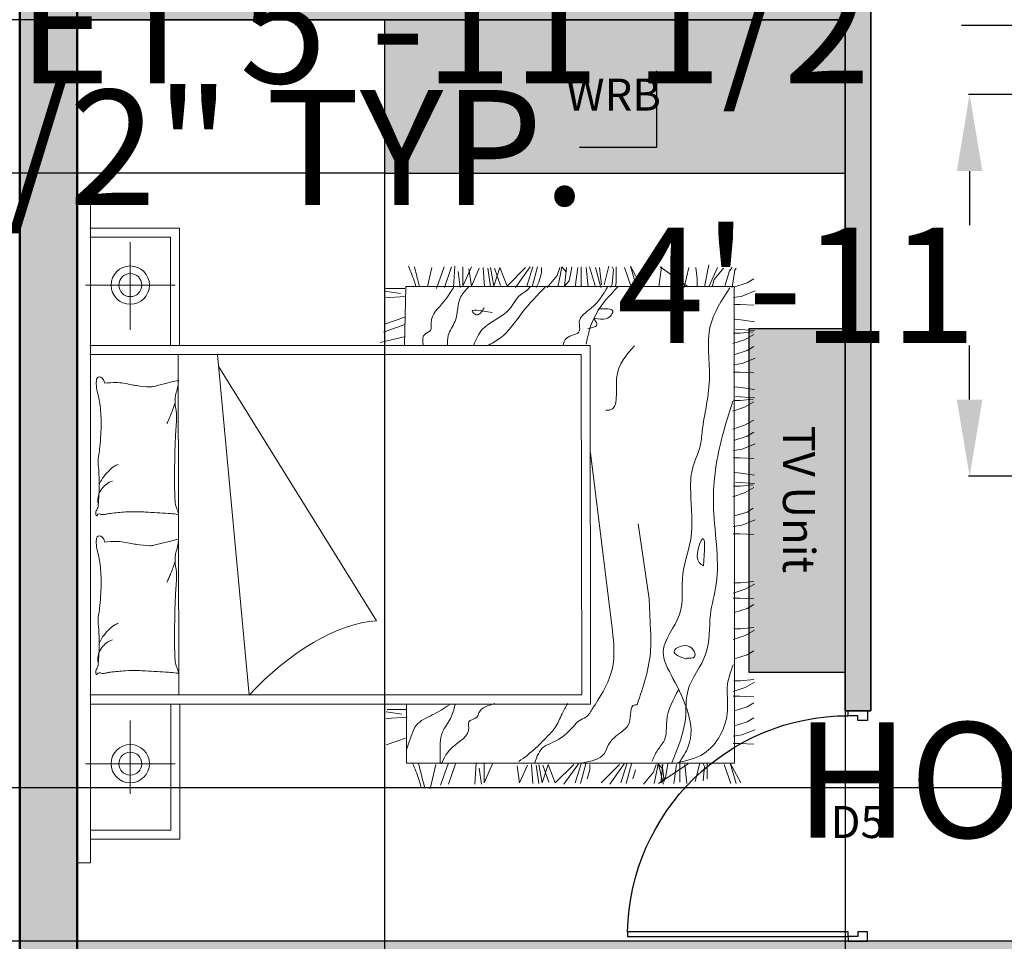
# Model space of a CAD drawing. Units: inches. Extents: x 2796 to 3603, y 978 to 1787.
# Tile 8 of 15: x 3070 to 3224, y 1312 to 1456. Entities that reach past the tile are written whole.
import ezdxf

# ---------------------------------------------------------------- set-up
doc = ezdxf.new("R2010")
doc.units = ezdxf.units.IN
for name, color, linetype, lineweight in [('A-ANNO-DIMS', 7, 'Continuous', 18), ('A-ANNO-TEXT', 7, 'Continuous', 18), ('A-DOOR', 6, 'Continuous', 25), ('A-FLOR-CASE', 2, 'Continuous', 25), ('A-FLOR-CASE-PATT', 2, 'Continuous', 13), ('A-WALL-EXTR-PATT', 1, 'Continuous', 13), ('A-WALL-INTR-PATT', 5, 'Continuous', 13), ('Furniture', 2, 'Continuous', 18), ('Inner Wall', 5, 'Continuous', 35), ('Outer Wall', 1, 'Continuous', 50)]:
    doc.layers.add(name, color=color, linetype=linetype, lineweight=lineweight)
doc.styles.get("Standard").update_dxf_attribs({"font": 'arial.ttf'})
doc.dimstyles.get("Standard").update_dxf_attribs({"dimtxt": 18, "dimasz": 12, "dimexe": 0.18, "dimexo": 0.0625, "dimgap": 0.09, "dimtad": 0, "dimtih": 1, "dimtoh": 1, "dimdec": 0, "dimzin": 0, "dimdsep": 46, "dimlunit": 3, "dimtxsty": 'Standard', "dimcen": 0.09, "dimadec": 0, "dimazin": 0, "dimtfac": 1, "dimtdec": 0, "dimtofl": 0, "dimtmove": 0, "dimatfit": 3, "dimfxl": 1, "dimtolj": 1, "dimtzin": 0, "dimarcsym": 0})

# ---------------------------------------------------------------- blocks, each defined once
blk = doc.blocks.new('A$C2B723114')
for p, q in [((0, 2.9047), (2.8274, 2.9047)), ((0, 2.8487), (0, 2.9047)), ((0.4243, 2.8697), (0.4243, 2.4855)), ((2.4742, 2.8697), (2.4742, 2.4855)), ((2.8274, 2.9047), (2.8274, 2.8487)), ((2.8274, 2.8487), (0, 2.8487)), ((0.1012, 2.4649), (0.1012, 2.849)), ((0.1396, 2.5033), (0.1396, 2.849)), ((0.6794, 0.7051), (0.6794, 2.8509)), ((0.7187, 0.7435), (0.7187, 2.8509)), ((2.1776, 2.8509), (2.1776, 0.7454)), ((2.216, 2.8509), (2.216, 0.707)), ((2.6798, 2.5052), (2.6798, 2.8509)), ((2.7182, 2.4668), (2.7182, 2.8509)), ((0.6087, 2.6776), (0.295, 2.6776)), ((2.6586, 2.6776), (2.2821, 2.6776)), ((1.3789, 2.4999), (1.3598, 2.5761)), ((2.0593, 2.4999), (2.0402, 2.5761)), ((0.6766, 2.5033), (0.1396, 2.5033)), ((1.3858, 2.4723), (1.3789, 2.4999)), ((2.0662, 2.4723), (2.0593, 2.4999)), ((2.2188, 2.5052), (2.6798, 2.5052)), ((0.6794, 2.4649), (0.1012, 2.4649)), ((0.7191, 2.47), (2.1778, 2.4719)), ((2.2188, 2.4668), (2.7182, 2.4668)), ((2.1771, 2.3036), (0.718, 2.1685)), ((1.0365, 1.6233), (2.1246, 2.2989)), ((2.2287, 1.6076), (2.2523, 1.5035)), ((0.5047, 1.5819), (0.5353, 1.4945)), ((0.6174, 1.5819), (0.6232, 1.4916)), ((0.6467, 1.5819), (0.6369, 1.5137)), ((0.6571, 1.4945), (0.6571, 1.5765)), ((2.2726, 1.593), (2.3061, 1.5007)), ((2.3067, 1.5881), (2.3373, 1.5007)), ((2.4194, 1.5881), (2.4251, 1.4979)), ((2.4487, 1.5881), (2.4389, 1.5199)), ((2.4591, 1.5007), (2.4591, 1.5828)), ((0.4269, 0.0884), (0.4269, 1.4945)), ((0.4269, 1.4945), (0.6794, 1.4945)), ((2.4685, 1.4964), (2.216, 1.5022)), ((2.4685, 1.4964), (2.4685, 0.0903)), ((0.3172, 1.3923), (0.4213, 1.3687)), ((2.4685, 1.4044), (2.5491, 1.3861)), ((2.4596, 1.3659), (2.552, 1.3324)), ((0.3318, 1.3485), (0.4241, 1.3149)), ((0.3367, 1.3143), (0.4241, 1.2838)), ((2.4645, 1.3318), (2.552, 1.3012)), ((2.4645, 1.2928), (2.5548, 1.2871)), ((2.4645, 1.2635), (2.5328, 1.2733)), ((2.4699, 1.2531), (2.552, 1.2163)), ((2.552, 1.2531), (2.4699, 1.2531)), ((2.5435, 1.2276), (2.4699, 1.2163)), ((0.3367, 1.2016), (0.427, 1.1959)), ((0.3367, 1.1724), (0.405, 1.1821)), ((2.4699, 1.2163), (2.5463, 1.1823)), ((0.4241, 1.162), (0.3421, 1.162)), ((0.3421, 1.162), (0.4241, 1.1252)), ((2.5491, 1.1654), (2.467, 1.1597)), ((2.5463, 1.1455), (2.467, 1.1342)), ((2.5491, 1.1342), (2.4699, 1.1201)), ((2.4699, 1.1201), (2.5491, 1.0946)), ((2.5463, 1.1172), (2.4727, 1.0918)), ((2.5491, 1.0946), (2.4699, 1.0635)), ((2.4699, 1.0635), (2.5491, 0.9842)), ((0.4157, 1.0206), (0.3421, 1.0093)), ((2.4642, 1.0267), (2.552, 0.9644)), ((0.3421, 1.0093), (0.4185, 0.9754)), ((2.4699, 0.9785), (2.552, 0.9531)), ((0.4213, 0.9584), (0.3392, 0.9527)), ((0.4185, 0.9386), (0.3392, 0.9272)), ((2.4642, 0.9389), (2.4869, 0.9276)), ((2.467, 0.9559), (2.552, 0.9333)), ((0.4213, 0.9272), (0.3421, 0.9131)), ((0.3421, 0.9131), (0.4213, 0.8876)), ((0.4213, 0.8876), (0.3421, 0.8565)), ((0.4185, 0.9103), (0.3449, 0.8848)), ((2.4642, 0.8908), (2.5152, 0.8483)), ((2.4869, 0.9276), (2.5265, 0.9163)), ((2.5265, 0.9163), (2.5491, 0.9163)), ((0.3421, 0.8565), (0.4213, 0.7772)), ((2.467, 0.8455), (2.5208, 0.8342)), ((2.5152, 0.8483), (2.5491, 0.837)), ((0.3364, 0.8197), (0.4241, 0.7574)), ((2.4699, 0.8172), (2.4925, 0.7974)), ((2.5491, 0.8087), (2.4699, 0.8172)), ((2.5208, 0.8342), (2.552, 0.8285)), ((2.552, 0.8285), (2.5293, 0.8087)), ((0.3421, 0.7716), (0.4241, 0.7461)), ((2.5491, 0.7606), (2.467, 0.7719)), ((2.4925, 0.7974), (2.535, 0.7889)), ((2.535, 0.7889), (2.552, 0.7861)), ((0.3392, 0.7489), (0.4241, 0.7263)), ((0.359, 0.7206), (0.3987, 0.7093)), ((2.1776, 0.7454), (0.7187, 0.7435)), ((2.4727, 0.7464), (2.467, 0.7408)), ((2.467, 0.7153), (2.5491, 0.7238)), ((2.552, 0.7464), (2.4727, 0.7464)), ((0.3987, 0.7093), (0.4213, 0.7093)), ((2.216, 0.707), (0.6794, 0.7051)), ((0.9938, 0.6115), (1.7555, 0.7064)), ((2.5491, 0.6842), (2.4642, 0.6615)), ((2.552, 0.7096), (2.467, 0.6842)), ((0.3421, 0.6601), (0.4213, 0.5808)), ((2.5491, 0.6672), (2.4755, 0.6587)), ((2.4755, 0.6474), (2.5548, 0.6276)), ((0.3364, 0.6233), (0.4241, 0.561)), ((2.4642, 0.6191), (2.4784, 0.6134)), ((2.467, 0.5993), (2.4869, 0.5964)), ((2.4784, 0.6134), (2.5406, 0.6077)), ((2.4869, 0.5964), (2.552, 0.5964)), ((2.5406, 0.6077), (2.552, 0.6134)), ((0.3392, 0.5525), (0.4241, 0.5299)), ((0.3421, 0.5752), (0.4241, 0.5497)), ((2.467, 0.5313), (2.5491, 0.5596)), ((0.359, 0.5242), (0.3987, 0.5129)), ((2.467, 0.5087), (2.5548, 0.5342)), ((2.5548, 0.5342), (2.4699, 0.4889)), ((0.3364, 0.4785), (0.3874, 0.436)), ((1.4523, 0.5021), (1.1305, 0.4537)), ((0.3392, 0.4332), (0.393, 0.4219)), ((0.3874, 0.436), (0.4213, 0.4247)), ((1.1305, 0.4537), (0.9938, 0.448)), ((0.4213, 0.415), (0.3364, 0.3923)), ((0.4241, 0.2868), (0.3392, 0.415)), ((0.3421, 0.4049), (0.3647, 0.3851)), ((0.4213, 0.3964), (0.3421, 0.4049)), ((0.4213, 0.398), (0.3477, 0.3895)), ((0.3647, 0.3851), (0.4072, 0.3766)), ((0.393, 0.4219), (0.4241, 0.4162)), ((0.4241, 0.4162), (0.4015, 0.3964)), ((2.467, 0.4133), (2.552, 0.4019)), ((2.467, 0.2879), (2.552, 0.4076)), ((0.4213, 0.3377), (0.3392, 0.3491)), ((0.4072, 0.3766), (0.4241, 0.3738)), ((0.3392, 0.2925), (0.4213, 0.3009)), ((0.4241, 0.3236), (0.3449, 0.3236)), ((2.4642, 0.3049), (2.5491, 0.2851)), ((2.467, 0.319), (2.5548, 0.3134)), ((0.3477, 0.2571), (0.427, 0.2373)), ((2.501, 0.2491), (2.5491, 0.2547)), ((0.3506, 0.2231), (0.4128, 0.2175)), ((0.4128, 0.2175), (0.4241, 0.2231)), ((2.467, 0.2179), (2.5605, 0.1981)), ((2.4699, 0.2491), (2.501, 0.2491)), ((0.359, 0.2061), (0.4241, 0.2061)), ((2.467, 0.1981), (2.5491, 0.1613)), ((2.467, 0.184), (2.4982, 0.1755)), ((2.4982, 0.1755), (2.5463, 0.1359)), ((0.3392, 0.1042), (0.4213, 0.1325)), ((2.4699, 0.1302), (2.535, 0.1104)), ((0.3392, 0.0815), (0.427, 0.107)), ((0.427, 0.107), (0.3421, 0.0617)), ((2.4685, 0.0903), (0.4269, 0.0884)), ((0.5106, 0.094), (0.5106, 0.0657)), ((0.5417, 0.094), (0.5474, 0.0572)), ((0.587, 0.0884), (0.604, 0.0346)), ((0.6512, 0.0884), (0.6682, 0.0346)), ((0.713, 0.094), (0.713, 0.0657)), ((0.7334, 0.0943), (0.7503, 0.0434)), ((0.7786, 0.0915), (0.7786, 0.0632)), ((0.8739, 0.0884), (0.8908, 0.0346)), ((0.956, 0.0943), (0.973, 0.0434)), ((1.0013, 0.0915), (1.0013, 0.0632)), ((1.072, 0.0884), (1.089, 0.0346)), ((1.1338, 0.094), (1.1338, 0.0657)), ((1.1542, 0.0943), (1.1712, 0.0434)), ((1.1995, 0.0915), (1.1995, 0.0632)), ((1.4088, 0.094), (1.4088, 0.0657)), ((1.44, 0.094), (1.4456, 0.0572)), ((1.4853, 0.0884), (1.5023, 0.0346)), ((1.5674, 0.0962), (1.5844, 0.0453)), ((1.6127, 0.0934), (1.6127, 0.0651)), ((1.6297, 0.0849), (1.624, 0.0028)), ((1.6721, 0.0877), (1.6693, 0.0623)), ((1.7344, 0.0934), (1.7344, 0.0651)), ((1.7655, 0.0934), (1.7712, 0.0566)), ((1.8108, 0.0877), (1.8278, 0.034)), ((1.8568, 0.0962), (1.8738, 0.0453)), ((1.9342, 0.0962), (1.9512, 0.0453)), ((1.9795, 0.0934), (1.9795, 0.0651)), ((1.9965, 0.0849), (1.9908, 0.0028)), ((2.039, 0.0877), (2.0361, 0.0623)), ((2.1012, 0.0934), (2.1012, 0.0651)), ((2.1324, 0.0934), (2.138, 0.0566)), ((2.1777, 0.0877), (2.1946, 0.034)), ((2.2236, 0.0962), (2.2406, 0.0453)), ((2.2689, 0.0934), (2.2689, 0.0651)), ((2.2859, 0.0849), (2.2802, 0.0028)), ((2.3284, 0.0877), (2.3255, 0.0623)), ((2.3906, 0.0934), (2.3906, 0.0651)), ((2.4218, 0.0934), (2.4274, 0.0566)), ((2.4642, 0.0991), (2.5378, 0.0877)), ((2.467, 0.0877), (2.484, 0.034)), ((2.535, 0.1104), (2.5491, 0.0991)), ((2.5378, 0.0877), (2.5463, 0.0821)), ((0.5106, 0.0657), (0.5077, 0.0063)), ((0.5474, 0.0572), (0.57, 0.0006)), ((0.713, 0.0657), (0.7101, 0.0063)), ((0.7503, 0.0434), (0.773, 0.0037)), ((0.7786, 0.0632), (0.7843, 0.0066)), ((0.973, 0.0434), (0.9957, 0.0037)), ((1.0013, 0.0632), (1.007, 0.0066)), ((1.1338, 0.0657), (1.131, 0.0063)), ((1.1712, 0.0434), (1.1939, 0.0037)), ((1.1995, 0.0632), (1.2052, 0.0066)), ((1.4088, 0.0657), (1.406, 0.0063)), ((1.4456, 0.0572), (1.4683, 0.0006)), ((1.5844, 0.0453), (1.607, 0.0057)), ((1.6127, 0.0651), (1.6184, 0.0085)), ((1.6693, 0.0623), (1.6608, 0.0028)), ((1.7344, 0.0651), (1.7316, 0.0057)), ((1.7712, 0.0566), (1.7938, 0)), ((1.8738, 0.0453), (1.8964, 0.0057)), ((1.9512, 0.0453), (1.9739, 0.0057)), ((1.9795, 0.0651), (1.9852, 0.0085)), ((2.0361, 0.0623), (2.0276, 0.0028)), ((2.1012, 0.0651), (2.0984, 0.0057)), ((2.138, 0.0566), (2.1607, 0)), ((2.2406, 0.0453), (2.2632, 0.0057)), ((2.2689, 0.0651), (2.2746, 0.0085)), ((2.3255, 0.0623), (2.317, 0.0028)), ((2.3906, 0.0651), (2.3878, 0.0057)), ((2.4274, 0.0566), (2.4501, 0)), ((0.604, 0.0346), (0.621, 0.0063)), ((0.6682, 0.0346), (0.6851, 0.0063)), ((0.8908, 0.0346), (0.9078, 0.0063)), ((1.089, 0.0346), (1.106, 0.0063)), ((1.5023, 0.0346), (1.5192, 0.0082)), ((1.8278, 0.034), (1.8448, 0.0057)), ((2.1946, 0.034), (2.2116, 0.0057)), ((2.484, 0.034), (2.501, 0.0057))]:
    blk.add_line(p, q)
for centre, radius in [((0.4243, 2.6776), 0.0821), ((2.4742, 2.6776), 0.0821), ((0.4243, 2.6776), 0.0493), ((2.4742, 2.6776), 0.0493)]:
    blk.add_circle(centre, radius)
for centre, radius, start, end in [((0.8078, 2.821), 0.00214, 160.436, 281.8931), ((0.8088, 2.8207), 0.00315, 111.7883, 160.436), ((0.8162, 2.8021), 0.0232, 94.3025, 111.7883), ((0.8091, 2.8151), 0.00394, 21.9904, 101.8931), ((0.8409, 2.7949), 0.0302, 158.579, 188.1335), ((1.0356, 2.8227), 0.2268, 188.1335, 192.1095), ((0.7994, 2.8112), 0.0144, 338.579, 21.9904), ((0.8165, 2.7987), 0.0266, 59.3487, 94.3025), ((0.8554, 2.8643), 0.0497, 239.3487, 264.7408), ((0.9202, 3.5684), 0.7568, 264.7408, 268.0921), ((0.8679, 2.7254), 0.0915, 74.0648, 94.2159), ((0.8679, 2.7254), 0.0915, 53.9136, 74.0648), ((0.9409, 4.189), 1.3777, 268.0921, 270.5757), ((0.8679, 2.7254), 0.0915, 36.1766, 53.9136), ((0.86, 2.6097), 0.2158, 62.7604, 69.1397), ((0.9466, 3.6164), 0.8051, 270.5757, 274.8018), ((0.9263, 2.7386), 0.0708, 51.6114, 62.7604), ((0.7461, 2.511), 0.3611, 46.1885, 51.6114), ((1.0364, 2.548), 0.2671, 87.4614, 94.8018), ((1.042, 2.6745), 0.1405, 79.8101, 87.4614), ((1.1532, 3.2931), 0.488, 259.8101, 263.9133), ((1.204, 3.7695), 0.9671, 263.9133, 270), ((1.204, 3.4318), 0.6294, 270, 277.5469), ((1.2573, 3.0292), 0.2233, 277.5469, 285.744), ((1.3941, 2.5438), 0.281, 98.4372, 105.744), ((1.3747, 2.6748), 0.1486, 90, 98.4372), ((1.3713, 2.8186), 0.0315, 274.4002, 333.4195), ((0.923, 2.7382), 0.4535, 0, 6.2324), ((1.3747, 2.74), 0.0833, 78.7276, 90), ((1.3886, 2.8099), 0.0121, 333.4195, 78.7276), ((1.4882, 2.821), 0.00214, 160.436, 281.8931), ((1.4892, 2.8207), 0.00315, 111.7883, 160.436), ((1.4966, 2.8021), 0.0232, 94.3025, 111.7883), ((1.4895, 2.8151), 0.00394, 21.9904, 101.8931), ((1.5213, 2.7949), 0.0302, 158.579, 188.1335), ((1.716, 2.8227), 0.2268, 188.1335, 192.1095), ((1.4798, 2.8112), 0.0144, 338.579, 21.9904), ((1.4969, 2.7987), 0.0266, 59.3487, 94.3025), ((1.5358, 2.8643), 0.0497, 239.3487, 264.7408), ((1.6006, 3.5684), 0.7568, 264.7408, 268.0921), ((1.5483, 2.7254), 0.0915, 74.0648, 94.2159), ((1.5483, 2.7254), 0.0915, 53.9136, 74.0648), ((1.6213, 4.189), 1.3777, 268.0921, 270.5757), ((1.5483, 2.7254), 0.0915, 36.1766, 53.9136), ((1.5404, 2.6097), 0.2158, 62.7604, 69.1397), ((1.627, 3.6164), 0.8051, 270.5757, 274.8018), ((1.6067, 2.7386), 0.0708, 51.6114, 62.7604), ((1.4265, 2.511), 0.3611, 46.1885, 51.6114), ((1.7168, 2.548), 0.2671, 87.4614, 94.8018), ((1.7224, 2.6745), 0.1405, 79.8101, 87.4614), ((1.8336, 3.2931), 0.488, 259.8101, 263.9133), ((1.8844, 3.7695), 0.9671, 263.9133, 270), ((1.8844, 3.4318), 0.6294, 270, 277.5469), ((1.9377, 3.0292), 0.2233, 277.5469, 285.744), ((2.0745, 2.5438), 0.281, 98.4372, 105.744), ((2.0551, 2.6748), 0.1486, 90, 98.4372), ((2.0517, 2.8186), 0.0315, 274.4002, 333.4195), ((1.6034, 2.7382), 0.4535, 0, 6.2324), ((2.0551, 2.74), 0.0833, 78.7276, 90), ((2.069, 2.8099), 0.0121, 333.4195, 78.7276), ((0.635, 2.7368), 0.1829, 7.6809, 12.1095), ((-0.0181, 2.6487), 0.8418, 3.3687, 7.6809), ((0.8679, 2.7254), 0.0915, 18.4397, 36.1766), ((0.8523, 2.6218), 0.2076, 39.0349, 46.1885), ((0.9783, 2.7239), 0.0455, 28.3168, 39.0349), ((0.8558, 2.6579), 0.1846, 23.0028, 28.3168), ((1.3154, 2.7368), 0.1829, 7.6809, 12.1095), ((0.6623, 2.6487), 0.8418, 3.3687, 7.6809), ((1.5483, 2.7254), 0.0915, 18.4397, 36.1766), ((1.5327, 2.6218), 0.2076, 39.0349, 46.1885), ((1.6587, 2.7239), 0.0455, 28.3168, 39.0349), ((1.5362, 2.6579), 0.1846, 23.0028, 28.3168), ((0.5722, 2.8434), 0.8132, 347.8016, 350.3156), ((1.1884, 2.7382), 0.1881, 350.3156, 0), ((1.2526, 2.8434), 0.8132, 347.8016, 350.3156), ((1.8688, 2.7382), 0.1881, 350.3156, 0), ((0.1976, 2.6614), 0.6258, 358.3669, 3.3687), ((1.6528, 2.6098), 0.2924, 167.8016, 171.9949), ((0.878, 2.6614), 0.6258, 358.3669, 3.3687), ((2.3332, 2.6098), 0.2924, 167.8016, 171.9949), ((-0.4351, 2.6794), 1.2587, 356.945, 358.3669), ((1.9648, 2.5659), 0.6074, 171.9949, 177.3351), ((0.2453, 2.6794), 1.2587, 356.945, 358.3669), ((2.6452, 2.5659), 0.6074, 171.9949, 177.3351), ((-11.7321, 3.2823), 12.5718, 356.49514, 356.94504), ((1.4204, 2.5912), 0.0624, 177.3351, 194.0452), ((-11.0517, 3.2823), 12.5718, 356.49514, 356.94504), ((2.1008, 2.5912), 0.0624, 177.3351, 194.0452), ((0.5206, 2.5319), 0.2961, 350.0016, 356.4951), ((1.4917, 3.1364), 0.681, 244.6889, 246.5156), ((1.4917, 3.1364), 0.681, 246.5156, 248.3423), ((1.4917, 3.1364), 0.681, 248.3423, 250.572), ((1.4917, 3.1364), 0.681, 250.572, 252.8018), ((1.201, 2.5319), 0.2961, 350.0016, 356.4951), ((2.1721, 3.1364), 0.681, 244.6889, 246.5156), ((2.1721, 3.1364), 0.681, 246.5156, 248.3423), ((2.1721, 3.1364), 0.681, 248.3423, 250.572), ((2.1721, 3.1364), 0.681, 250.572, 252.8018), ((0.8298, 2.4774), 0.0178, 170.0016, 196.6978), ((0.8139, 2.4726), 0.00122, 196.6978, 277.1204), ((0.8041, 2.5514), 0.0807, 277.1204, 286.2212), ((0.8068, 2.5419), 0.0707, 286.2212, 297.2841), ((0.8584, 2.4419), 0.0418, 102.869, 117.2841), ((0.879, 2.3515), 0.1345, 93.574, 102.869), ((0.9376, 1.4146), 1.0732, 90.2865, 93.574), ((0.9586, -2.7845), 5.2724, 89.0296, 90.2865), ((0.9954, -0.6123), 3.0999, 87.3904, 89.0296), ((1.0854, 1.364), 1.1216, 85.3824, 87.3904), ((1.28, 3.7729), 1.2952, 265.3824, 267.2509), ((1.228, 2.691), 0.2121, 267.2509, 281.5586), ((1.2975, 2.3514), 0.1345, 83.5659, 101.5586), ((1.3002, 2.3754), 0.1104, 72.6136, 83.5659), ((1.3965, 2.6828), 0.2118, 252.6136, 260.5159), ((1.4027, 2.7202), 0.2496, 260.5159, 265.9171), ((1.385, 2.4721), 0.000845, 265.9171, 14.0449), ((1.5102, 2.4774), 0.0178, 170.0016, 196.6978), ((1.4943, 2.4726), 0.00122, 196.6978, 277.1204), ((1.4845, 2.5514), 0.0807, 277.1204, 286.2212), ((1.4872, 2.5419), 0.0707, 286.2212, 297.2841), ((1.5388, 2.4419), 0.0418, 102.869, 117.2841), ((1.5594, 2.3515), 0.1345, 93.574, 102.869), ((1.618, 1.4146), 1.0732, 90.2865, 93.574), ((1.639, -2.7845), 5.2724, 89.0296, 90.2865), ((1.6758, -0.6123), 3.0999, 87.3904, 89.0296), ((1.7658, 1.364), 1.1216, 85.3824, 87.3904), ((1.9604, 3.7729), 1.2952, 265.3824, 267.2509), ((1.9084, 2.691), 0.2121, 267.2509, 281.5586), ((1.9779, 2.3514), 0.1345, 83.5659, 101.5586), ((1.9806, 2.3754), 0.1104, 72.6136, 83.5659), ((2.0769, 2.6828), 0.2118, 252.6136, 260.5159), ((2.0831, 2.7202), 0.2496, 260.5159, 265.9171), ((2.0654, 2.4721), 0.000845, 265.9171, 14.0449)]:
    blk.add_arc(centre, radius, start, end)
blk.add_ellipse((0.4962, 1.9132), major_axis=(0.4887, -0.4605), ratio=0.503305, start_param=0.491272, end_param=1.591113)
for points, knots in [([(0.6768, 1.3104), (0.6615, 1.3339), (0.6315, 1.3797), (0.604, 1.4501), (0.5417, 1.4748), (0.5064, 1.4871), (0.4848, 1.4945)], [0, 0, 0, 0, 110.980521, 216.571322, 273.316778, 363.252298, 363.252298, 363.252298, 363.252298]), ([(2.5548, 1.4853), (2.5314, 1.4757), (2.5031, 1.4641), (2.4737, 1.4555), (2.4685, 1.454)], [0, 0, 0, 0, 98.452083, 119.481049, 119.481049, 119.481049, 119.481049]), ([(0.427, 1.4678), (0.4036, 1.4582), (0.3693, 1.4441), (0.3335, 1.4344), (0.3221, 1.4313)], [0, 0, 0, 0, 98.452083, 144.639601, 144.639601, 144.639601, 144.639601]), ([(0.4241, 1.4423), (0.4031, 1.437), (0.3691, 1.4284), (0.3351, 1.4199), (0.3221, 1.4167)], [0, 0, 0, 0, 84.638756, 136.955563, 136.955563, 136.955563, 136.955563]), ([(2.552, 1.4598), (2.5309, 1.4545), (2.5031, 1.4475), (2.4753, 1.4406), (2.4685, 1.4389)], [0, 0, 0, 0, 84.638756, 111.94623, 111.94623, 111.94623, 111.94623]), ([(2.2145, 1.4211), (2.233, 1.4246), (2.2636, 1.4303), (2.2761, 1.3837), (2.3429, 1.3967), (2.3949, 1.3342), (2.4474, 1.3031), (2.4698, 1.2898)], [0, 0, 0, 0, 61.886907, 102.717887, 145.699352, 284.082577, 386.765171, 386.765171, 386.765171, 386.765171]), ([(0.6768, 1.286), (0.6567, 1.2911), (0.6145, 1.3017), (0.5543, 1.3533), (0.4816, 1.349), (0.4362, 1.3493), (0.4233, 1.3493)], [0, 0, 0, 0, 80.250278, 168.388677, 295.908361, 346.663112, 346.663112, 346.663112, 346.663112]), ([(0.4233, 1.3445), (0.4367, 1.3385), (0.464, 1.3264), (0.5129, 1.2848), (0.5456, 1.2161), (0.6131, 1.2349), (0.6142, 1.1913), (0.6642, 1.1806), (0.674, 1.144), (0.6817, 1.1154)], [0, 0, 0, 0, 56.745495, 115.23739, 254.956954, 286.678662, 337.828324, 366.201072, 468.500395, 468.500395, 468.500395, 468.500395]), ([(2.2145, 1.319), (2.2295, 1.319), (2.2678, 1.3192), (2.3288, 1.2705), (2.4143, 1.279), (2.4535, 1.2403), (2.4662, 1.2278)], [0, 0, 0, 0, 57.155505, 146.33427, 287.936209, 355.396728, 355.396728, 355.396728, 355.396728]), ([(2.3573, 1.127), (2.3656, 1.1759), (2.3758, 1.2352), (2.3371, 1.1853), (2.3602, 1.1713), (2.3768, 1.1612)], [0, 0, 0, 0, 107.853607, 130.728419, 189.220329, 189.220329, 189.220329, 189.220329]), ([(2.2182, 1.2059), (2.2419, 1.1958), (2.3116, 1.1659), (2.342, 1.0552), (2.4266, 1.0223), (2.4474, 0.9811), (2.462, 0.9684), (2.4698, 0.9616)], [0, 0, 0, 0, 97.73655, 287.59661, 389.176293, 423.403759, 463.679181, 463.679181, 463.679181, 463.679181]), ([(2.2145, 1.1476), (2.2246, 1.1286), (2.2575, 1.0666), (2.3612, 1.0009), (2.431, 0.9336), (2.4662, 0.8996)], [0, 0, 0, 0, 83.02987, 271.460712, 463.033803, 463.033803, 463.033803, 463.033803]), ([(0.6817, 0.8034), (0.6673, 0.8119), (0.6341, 0.8315), (0.5785, 0.8518), (0.5349, 0.8973), (0.4828, 0.9461), (0.4518, 0.9879), (0.4331, 1.013)], [0, 0, 0, 0, 65.318952, 150.437229, 226.833166, 307.58338, 429.454095, 429.454095, 429.454095, 429.454095]), ([(0.4282, 0.9448), (0.4547, 0.9353), (0.496, 0.9206), (0.5223, 0.8436), (0.5628, 0.7946), (0.6113, 0.7575), (0.6214, 0.7173), (0.6539, 0.7022), (0.672, 0.6897), (0.6768, 0.6864)], [0, 0, 0, 0, 102.299436, 159.044876, 303.717955, 348.579152, 391.138254, 454.581655, 477.456496, 477.456496, 477.456496, 477.456496]), ([(2.2145, 0.823), (2.227, 0.8201), (2.261, 0.8121), (2.261, 0.7401), (2.3352, 0.7659), (2.379, 0.6836), (2.4336, 0.6521), (2.4662, 0.6334)], [0, 0, 0, 0, 46.747668, 127.438174, 179.649794, 280.561838, 429.605131, 429.605131, 429.605131, 429.605131]), ([(0.4282, 0.74), (0.4347, 0.7029), (0.444, 0.6496), (0.5194, 0.6274), (0.555, 0.5807), (0.5975, 0.5243), (0.6789, 0.5415), (0.677, 0.5095), (0.6768, 0.5061)], [0, 0, 0, 0, 130.791737, 187.537266, 286.231946, 353.673191, 460.023761, 472.712403, 472.712403, 472.712403, 472.712403]), ([(2.2218, 0.7246), (2.2595, 0.716), (2.3548, 0.6945), (2.4265, 0.6268), (2.4698, 0.586)], [0, 0, 0, 0, 148.665024, 375.555892, 375.555892, 375.555892, 375.555892]), ([(2.3719, 0.6737), (2.3738, 0.6431), (2.3772, 0.5878), (2.3146, 0.6382), (2.3401, 0.7015), (2.2971, 0.6649), (2.2923, 0.6965), (2.289, 0.7176)], [0, 0, 0, 0, 83.446591, 150.887818, 201.642461, 230.015204, 286.760644, 286.760644, 286.760644, 286.760644]), ([(0.6768, 0.6864), (0.7275, 0.655), (0.8251, 0.5944), (0.9391, 0.606), (0.9938, 0.6115)], [0, 0, 0, 0, 225.995823, 434.686543, 434.686543, 434.686543, 434.686543]), ([(2.2145, 0.5167), (2.1764, 0.5522), (2.1051, 0.6184), (1.9357, 0.5803), (1.9385, 0.6342), (1.9388, 0.6395)], [0, 0, 0, 0, 208.073343, 389.01094, 409.01094, 409.01094, 409.01094, 409.01094]), ([(0.6768, 0.5061), (0.7554, 0.4794), (0.8591, 0.4442), (0.9675, 0.4473), (0.9938, 0.448)], [0, 0, 0, 0, 319.374611, 421.61723, 421.61723, 421.61723, 421.61723]), ([(0.4331, 0.4427), (0.4498, 0.4356), (0.4827, 0.4216), (0.5314, 0.3759), (0.632, 0.3884), (0.6996, 0.3513), (0.7423, 0.3278)], [0, 0, 0, 0, 70.931849, 139.556414, 248.154027, 434.709995, 434.709995, 434.709995, 434.709995]), ([(2.4625, 0.1088), (2.4095, 0.1438), (2.2904, 0.2226), (2.0623, 0.1771), (1.9006, 0.2246), (1.7699, 0.2337), (1.6941, 0.2766), (1.5528, 0.2786), (1.4005, 0.2587), (1.2324, 0.3267), (1.059, 0.2939), (0.9218, 0.426), (0.7359, 0.3204), (0.5586, 0.2391), (0.4502, 0.3116), (0.427, 0.3272)], [0, 0, 0, 0, 239.874704, 538.942419, 850.40885, 893.390315, 1047.998294, 1176.505142, 1437.500972, 1637.333004, 1864.324391, 2089.058767, 2248.736533, 2637.953392, 2744.252142, 2744.252142, 2744.252142, 2744.252142]), ([(1.9771, 0.0962), (1.9286, 0.1117), (1.7864, 0.157), (1.5223, 0.1992), (1.2611, 0.141), (1.0527, 0.2023), (0.8859, 0.1885), (0.76, 0.3042), (0.6211, 0.292), (0.5187, 0.3203), (0.4572, 0.3456), (0.4282, 0.3575)], [0, 0, 0, 0, 198.710624, 582.73994, 1031.873213, 1206.082894, 1423.278209, 1655.952104, 1808.744089, 1945.69963, 2068.229211, 2068.229211, 2068.229211, 2068.229211]), ([(0.8718, 0.2941), (0.8821, 0.3221), (0.9041, 0.3814), (0.9523, 0.2773), (0.8733, 0.2454), (0.8757, 0.2798), (0.8766, 0.2941)], [0, 0, 0, 0, 82.720021, 175.094899, 237.579423, 282.440623, 282.440623, 282.440623, 282.440623]), ([(0.8474, 0.0943), (0.82, 0.1047), (0.757, 0.1287), (0.6201, 0.1029), (0.4623, 0.1837), (0.4372, 0.2936), (0.4282, 0.3331)], [0, 0, 0, 0, 112.422038, 258.341957, 533.791494, 688.286079, 688.286079, 688.286079, 688.286079]), ([(1.2715, 0.221), (1.3344, 0.2172), (1.4529, 0.21), (1.2971, 0.2665), (1.2756, 0.2284), (1.2715, 0.221)], [0, 0, 0, 0, 150.888188, 283.977876, 315.699589, 315.699589, 315.699589, 315.699589])]:
    blk.add_open_spline(points, degree=3, knots=knots)
blk = doc.blocks.new('*D12')
at = {"layer": 'A-ANNO-DIMS', "color": 0, "lineweight": -2, "transparency": 16777216}
for p, q in [((3070.18, 1736.68), (3041.33, 1736.68)), ((3041.51, 1724.68), (3041.51, 1391.96)), ((3041.51, 1040.68), (3041.51, 1373.4)), ((3070.18, 1028.68), (3041.33, 1028.68))]:
    blk.add_line(p, q, dxfattribs=at)
at = {"layer": 'A-ANNO-DIMS', "color": 0, "transparency": 16777216}
for points in [[(3039.51, 1724.68), (3043.51, 1724.68), (3041.51, 1736.68)], [(3039.51, 1040.68), (3043.51, 1040.68), (3041.51, 1028.68)]]:
    blk.add_solid(points, dxfattribs=at)
at = {"layer": 'Defpoints', "color": 0, "transparency": 16777216}
for p in [(3041.51, 1736.68), (3070.25, 1736.68), (3070.25, 1028.68)]:
    blk.add_point(p, dxfattribs=at)
at = {"layer": 'A-ANNO-DIMS', "color": 0, "transparency": 16777216, "insert": (3041.51, 1382.68), "char_height": 18, "attachment_point": 5}
blk.add_mtext("\\A1;59'", dxfattribs=at)
blk = doc.blocks.new('DOOR-SWING-36IN')
for points in [[(-0.01, 34.5), (-0.01, 0), (-0.76, 0), (-0.76, 34.5)], [(-35.26, -3), (-33.76, -3), (-33.76, -1.5), (-34.51, -1.5), (-34.51, 0), (-35.26, 0)], [(0.74, -3), (-0.76, -3), (-0.76, -1.5), (-0.01, -1.5), (-0.01, 0), (0.74, 0)]]:
    blk.add_lwpolyline(points, close=True)
blk.add_arc((0, 0), 34.51, 91.2592, 180)
blk = doc.blocks.new('*D22')
at = {"layer": 'A-ANNO-DIMS', "color": 0, "lineweight": -2, "transparency": 16777216}
for p, q in [((3160.28, 1475.52), (3148.28, 1475.52)), ((3172.28, 1473.07), (3172.28, 1475.7)), ((3189.07, 1473.07), (3189.07, 1475.7)), ((3201.07, 1475.52), (3213.07, 1475.52))]:
    blk.add_line(p, q, dxfattribs=at)
at = {"layer": 'A-ANNO-DIMS', "color": 0, "transparency": 16777216}
for points in [[(3160.28, 1477.52), (3160.28, 1473.52), (3172.28, 1475.52)], [(3201.07, 1477.52), (3201.07, 1473.52), (3189.07, 1475.52)]]:
    blk.add_solid(points, dxfattribs=at)
at = {"layer": 'Defpoints', "color": 0, "transparency": 16777216}
for p in [(3172.28, 1475.52), (3172.28, 1473), (3189.07, 1473)]:
    blk.add_point(p, dxfattribs=at)
at = {"layer": 'A-ANNO-DIMS', "color": 0, "transparency": 16777216, "insert": (3052.51, 1475.52), "char_height": 18, "attachment_point": 5}
blk.add_mtext('\\A1;BASIN 1\'-5" TYP.', dxfattribs=at)
blk = doc.blocks.new('*D23')
at = {"layer": 'A-ANNO-DIMS', "color": 0, "lineweight": -2, "transparency": 16777216}
for p, q in [((3169.76, 1485), (3169.76, 1497)), ((3172.22, 1473), (3169.58, 1473)), ((3172.22, 1459.7), (3169.58, 1459.7)), ((3169.76, 1447.7), (3169.76, 1435.7)), ((3169.76, 1435.7), (3157.76, 1435.7))]:
    blk.add_line(p, q, dxfattribs=at)
at = {"layer": 'A-ANNO-DIMS', "color": 0, "transparency": 16777216}
for points in [[(3167.76, 1485), (3171.76, 1485), (3169.76, 1473)], [(3167.76, 1447.7), (3171.76, 1447.7), (3169.76, 1459.7)]]:
    blk.add_solid(points, dxfattribs=at)
at = {"layer": 'Defpoints', "color": 0, "transparency": 16777216}
for p in [(3172.28, 1473), (3169.76, 1459.7), (3172.28, 1459.7)]:
    blk.add_point(p, dxfattribs=at)
at = {"layer": 'A-ANNO-DIMS', "color": 0, "transparency": 16777216, "insert": (3082.69, 1435.7), "char_height": 18, "attachment_point": 5}
blk.add_mtext('\\A1;1\'-1 1/2" TYP.', dxfattribs=at)
blk = doc.blocks.new('*D32')
at = {"layer": 'A-ANNO-DIMS', "color": 0, "lineweight": -2, "transparency": 16777216}
for p, q in [((3229.46, 1454.75), (3217.46, 1454.75)), ((3229.46, 1444.07), (3229.46, 1454.93)), ((3289.09, 1454.75), (3241.46, 1454.75)), ((3301.09, 1444.07), (3301.09, 1454.93))]:
    blk.add_line(p, q, dxfattribs=at)
at = {"layer": 'A-ANNO-DIMS', "color": 0, "transparency": 16777216}
for points in [[(3241.46, 1456.75), (3241.46, 1452.75), (3229.46, 1454.75)], [(3289.09, 1456.75), (3289.09, 1452.75), (3301.09, 1454.75)]]:
    blk.add_solid(points, dxfattribs=at)
at = {"layer": 'Defpoints', "color": 0, "transparency": 16777216}
for p in [(3229.46, 1454.75), (3229.46, 1444.01), (3301.09, 1444.01)]:
    blk.add_point(p, dxfattribs=at)
at = {"layer": 'A-ANNO-DIMS', "color": 0, "transparency": 16777216, "insert": (3090.48, 1454.75), "char_height": 18, "attachment_point": 5}
blk.add_mtext('\\A1;DINING SET 5\'-11 1/2"', dxfattribs=at)
blk = doc.blocks.new('*D33')
at = {"layer": 'A-ANNO-DIMS', "color": 0, "lineweight": -2, "transparency": 16777216}
for p, q in [((3229.39, 1444.01), (3218.53, 1444.01)), ((3218.71, 1432.01), (3218.71, 1423.57)), ((3218.71, 1396.33), (3218.71, 1404.77)), ((3229.39, 1384.33), (3218.53, 1384.33))]:
    blk.add_line(p, q, dxfattribs=at)
at = {"layer": 'A-ANNO-DIMS', "color": 0, "transparency": 16777216}
for points in [[(3216.71, 1432.01), (3220.71, 1432.01), (3218.71, 1444.01)], [(3216.71, 1396.33), (3220.71, 1396.33), (3218.71, 1384.33)]]:
    blk.add_solid(points, dxfattribs=at)
at = {"layer": 'Defpoints', "color": 0, "transparency": 16777216}
for p in [(3229.46, 1444.01), (3218.71, 1384.33), (3229.46, 1384.33)]:
    blk.add_point(p, dxfattribs=at)
at = {"layer": 'A-ANNO-DIMS', "color": 0, "transparency": 16777216, "insert": (3218.71, 1414.17), "char_height": 18, "attachment_point": 5}
blk.add_mtext('\\A1;4\'-11 1/2"', dxfattribs=at)
blk = doc.blocks.new('*D34')
at = {"layer": 'A-ANNO-DIMS', "color": 0, "lineweight": -2, "transparency": 16777216}
for p, q in [((3355.83, 1336.87), (3343.83, 1336.87)), ((3355.83, 1332.81), (3355.83, 1337.05)), ((3371.32, 1336.87), (3367.83, 1336.87)), ((3383.32, 1332.81), (3383.32, 1337.05))]:
    blk.add_line(p, q, dxfattribs=at)
at = {"layer": 'A-ANNO-DIMS', "color": 0, "transparency": 16777216}
for points in [[(3367.83, 1338.87), (3367.83, 1334.87), (3355.83, 1336.87)], [(3371.32, 1338.87), (3371.32, 1334.87), (3383.32, 1336.87)]]:
    blk.add_solid(points, dxfattribs=at)
at = {"layer": 'Defpoints', "color": 0, "transparency": 16777216}
for p in [(3355.83, 1336.87), (3355.83, 1332.75), (3383.32, 1332.75)]:
    blk.add_point(p, dxfattribs=at)
at = {"layer": 'A-ANNO-DIMS', "color": 0, "transparency": 16777216, "insert": (3268.59, 1336.87), "char_height": 18, "attachment_point": 5}
blk.add_mtext('\\A1;HOB 2\'-3 1/2"', dxfattribs=at)
blk = doc.blocks.new('*D41')
at = {"layer": 'A-ANNO-DIMS', "color": 0, "lineweight": -2, "transparency": 16777216}
for p, q in [((3079.18, 1455.68), (3031.37, 1455.68)), ((3031.55, 1443.68), (3031.55, 1392.96)), ((3031.55, 1323.68), (3031.55, 1374.4)), ((3079.18, 1311.68), (3031.37, 1311.68))]:
    blk.add_line(p, q, dxfattribs=at)
at = {"layer": 'A-ANNO-DIMS', "color": 0, "transparency": 16777216}
for points in [[(3029.55, 1443.68), (3033.55, 1443.68), (3031.55, 1455.68)], [(3029.55, 1323.68), (3033.55, 1323.68), (3031.55, 1311.68)]]:
    blk.add_solid(points, dxfattribs=at)
at = {"layer": 'Defpoints', "color": 0, "transparency": 16777216}
for p in [(3031.55, 1455.68), (3079.25, 1455.68), (3079.25, 1311.68)]:
    blk.add_point(p, dxfattribs=at)
at = {"layer": 'A-ANNO-DIMS', "color": 0, "transparency": 16777216, "insert": (3031.55, 1383.68), "char_height": 18, "attachment_point": 5}
blk.add_mtext('\\A1;12\'-0"', dxfattribs=at)
blk = doc.blocks.new('*D51')
at = {"layer": 'A-ANNO-DIMS', "color": 0, "lineweight": -2, "transparency": 16777216}
for p, q in [((3127.245499, 1431.61284), (3127.245499, 989.79534)), ((3199.245499, 1431.61284), (3199.245499, 989.79534)), ((3115.245499, 989.97534), (3103.245499, 989.97534)), ((3211.245499, 989.97534), (3223.245499, 989.97534))]:
    blk.add_line(p, q, dxfattribs=at)
at = {"layer": 'A-ANNO-DIMS', "color": 0, "transparency": 16777216}
for points in [[(3115.245499, 991.97534), (3115.245499, 987.97534), (3127.245499, 989.97534)], [(3211.245499, 991.97534), (3211.245499, 987.97534), (3199.245499, 989.97534)]]:
    blk.add_solid(points, dxfattribs=at)
at = {"layer": 'Defpoints', "color": 0, "transparency": 16777216}
for p in [(3127.245499, 1431.67534), (3199.245499, 1431.67534), (3199.245499, 989.97534)]:
    blk.add_point(p, dxfattribs=at)
at = {"layer": 'A-ANNO-DIMS', "color": 0, "transparency": 16777216, "insert": (3163.245499, 989.97534), "char_height": 18, "attachment_point": 5}
blk.add_mtext('\\A1;6\'-0"', dxfattribs=at)
blk = doc.blocks.new('*D52')
at = {"layer": 'A-ANNO-DIMS', "color": 0, "lineweight": -2, "transparency": 16777216}
for p, q in [((3031.545499, 1467.67534), (3031.545499, 1479.67534)), ((3127.182999, 1455.67534), (3031.365499, 1455.67534)), ((3127.182999, 1431.67534), (3031.365499, 1431.67534)), ((3031.545499, 1419.67534), (3031.545499, 1407.67534))]:
    blk.add_line(p, q, dxfattribs=at)
at = {"layer": 'A-ANNO-DIMS', "color": 0, "transparency": 16777216}
for points in [[(3029.545499, 1467.67534), (3033.545499, 1467.67534), (3031.545499, 1455.67534)], [(3029.545499, 1419.67534), (3033.545499, 1419.67534), (3031.545499, 1431.67534)]]:
    blk.add_solid(points, dxfattribs=at)
at = {"layer": 'Defpoints', "color": 0, "transparency": 16777216}
for p in [(3031.545499, 1455.67534), (3127.245499, 1455.67534), (3127.245499, 1431.67534)]:
    blk.add_point(p, dxfattribs=at)
at = {"layer": 'A-ANNO-DIMS', "color": 0, "transparency": 16777216, "insert": (3031.545499, 1443.67534), "char_height": 18, "attachment_point": 5}
blk.add_mtext('\\A1;2\'-0"', dxfattribs=at)
blk = doc.blocks.new('*D53')
at = {"layer": 'A-ANNO-DIMS', "color": 0, "lineweight": -2, "transparency": 16777216}
for p, q in [((3031.545499, 1347.67534), (3031.545499, 1359.67534)), ((3333.182999, 1335.67534), (3031.365499, 1335.67534)), ((3333.182999, 1311.67534), (3031.365499, 1311.67534)), ((3031.545499, 1299.67534), (3031.545499, 1287.67534))]:
    blk.add_line(p, q, dxfattribs=at)
at = {"layer": 'A-ANNO-DIMS', "color": 0, "transparency": 16777216}
for points in [[(3029.545499, 1347.67534), (3033.545499, 1347.67534), (3031.545499, 1335.67534)], [(3029.545499, 1299.67534), (3033.545499, 1299.67534), (3031.545499, 1311.67534)]]:
    blk.add_solid(points, dxfattribs=at)
at = {"layer": 'Defpoints', "color": 0, "transparency": 16777216}
for p in [(3031.545499, 1335.67534), (3333.245499, 1335.67534), (3333.245499, 1311.67534)]:
    blk.add_point(p, dxfattribs=at)
at = {"layer": 'A-ANNO-DIMS', "color": 0, "transparency": 16777216, "insert": (3031.545499, 1323.67534), "char_height": 18, "attachment_point": 5}
blk.add_mtext('\\A1;2\'-0"', dxfattribs=at)

msp = doc.modelspace()

# ---------------------------------------------------------------- hatches: boundary and pattern name
at = {"layer": 'A-FLOR-CASE-PATT'}
h = msp.add_hatch(dxfattribs=at)
h.set_pattern_fill('GOST_WOOD', color=256)
h.paths.add_polyline_path([(3127.25, 1727.68), (3079.25, 1727.68), (3079.25, 1703.68), (3127.25, 1703.68)])
h.paths.add_polyline_path([(3245.25, 1629.3), (3230.25, 1629.3), (3230.25, 1563.53), (3245.25, 1563.53)])
h.paths.add_polyline_path([(3381.25, 1651.68), (3315.48, 1651.68), (3315.48, 1636.68), (3381.25, 1636.68)])
h.paths.add_polyline_path([(3415.25, 1603.68), (3391.25, 1603.68), (3391.25, 1507.68), (3415.25, 1507.68)])
h.paths.add_polyline_path([(3199.25, 1407.44), (3184.25, 1407.44), (3184.25, 1353.68), (3199.25, 1353.68)])
h.paths.add_polyline_path([(3199.25, 1455.68), (3127.25, 1455.68), (3127.25, 1431.68), (3199.25, 1431.68)])
h.paths.add_polyline_path([(3223.25, 1244.56), (3208.25, 1244.56), (3208.25, 1178.79), (3223.25, 1178.79)])
h.paths.add_polyline_path([(3093.36, 1710.13), (3112.68, 1710.13), (3112.68, 1720.81), (3093.36, 1720.81)], flags=24)
h.paths.add_polyline_path([(3232.57, 1610.37), (3232.57, 1583.04), (3243.25, 1583.04), (3243.25, 1610.37)], flags=24)
h.paths.add_polyline_path([(3334.41, 1639), (3361.73, 1639), (3361.73, 1649.68), (3334.41, 1649.68)], flags=24)
h.paths.add_polyline_path([(3398.2, 1565.36), (3398.2, 1546.04), (3408.87, 1546.04), (3408.87, 1565.36)], flags=24)
h.paths.add_polyline_path([(3186.57, 1394.51), (3186.57, 1367.19), (3197.25, 1367.19), (3197.25, 1394.51)], flags=24)
h.paths.add_polyline_path([(3153.56, 1438.63), (3172.88, 1438.63), (3172.88, 1449.3), (3153.56, 1449.3)], flags=24)
h.paths.add_polyline_path([(3210.57, 1225.63), (3210.57, 1198.3), (3221.25, 1198.3), (3221.25, 1225.63)], flags=24)
at = {"layer": 'A-WALL-EXTR-PATT'}
h = msp.add_hatch(color=256, dxfattribs=at)
h.dxf.hatch_style = 1
h.paths.add_polyline_path([(3424.25, 1736.68), (3070.25, 1736.68), (3070.25, 1106.68), (3227.25, 1106.68), (3227.25, 1115.68), (3226.75, 1115.68), (3223.75, 1115.68), (3079.25, 1115.68), (3079.25, 1727.68), (3127.25, 1727.68), (3415.25, 1727.68), (3415.25, 1188.68), (3424.25, 1188.68)])
h.paths.add_polyline_path([(3291.25, 1032.68), (3074.25, 1032.68), (3074.25, 1106.68), (3070.25, 1106.68), (3070.25, 1028.68), (3291.25, 1028.68)])
h.paths.add_polyline_path([(3291.25, 1115.68), (3281.25, 1115.68), (3281.25, 1106.68), (3291.25, 1106.68)], flags=17)
h.paths.add_polyline_path([(3301.25, 1037.68), (3291.25, 1037.68), (3291.25, 1028.68), (3301.25, 1028.68)])
h.paths.add_polyline_path([(3424.25, 1037.68), (3414.25, 1037.68), (3414.25, 1028.68), (3424.25, 1028.68)])
h.paths.add_polyline_path([(3424.25, 1188.68), (3420.25, 1188.68), (3420.25, 1037.68), (3424.25, 1037.68)])
at = {"layer": 'A-WALL-INTR-PATT'}
h = msp.add_hatch(color=256, dxfattribs=at)
h.dxf.hatch_style = 1
h.paths.add_polyline_path([(3249.25, 1727.68), (3245.25, 1727.68), (3245.25, 1655.68), (3103.25, 1655.68), (3103.25, 1651.68), (3245.25, 1651.68), (3245.25, 1503.68), (3249.25, 1503.68)])
h.paths.add_polyline_path([(3131.25, 1727.68), (3127.25, 1727.68), (3127.25, 1703.68), (3127.25, 1679.68), (3131.25, 1679.68)], flags=17)
h.paths.add_polyline_path([(3391.25, 1655.68), (3325.25, 1655.68), (3325.25, 1727.68), (3321.25, 1727.68), (3321.25, 1655.68), (3273.25, 1655.68), (3273.25, 1651.68), (3391.25, 1651.68)])
h.paths.add_polyline_path([(3203.25, 1459.68), (3079.25, 1459.68), (3079.25, 1455.68), (3199.25, 1455.68), (3199.25, 1431.68), (3199.25, 1347.68), (3203.25, 1347.68)])
h.paths.add_polyline_path([(3209.25, 1507.68), (3079.25, 1507.68), (3079.25, 1503.68), (3209.25, 1503.68)])
h.paths.add_polyline_path([(3415.25, 1507.68), (3285.25, 1507.68), (3285.25, 1503.68), (3415.25, 1503.68)])
h.paths.add_polyline_path([(3415.25, 1459.68), (3333.25, 1459.68), (3333.25, 1455.68), (3415.25, 1455.68)])
h.paths.add_polyline_path([(3291.25, 1311.68), (3287.25, 1311.68), (3287.25, 1192.68), (3227.25, 1192.68), (3227.25, 1267.68), (3263.25, 1267.68), (3263.25, 1271.68), (3223.25, 1271.68), (3223.25, 1151.68), (3227.25, 1151.68), (3227.25, 1188.68), (3291.25, 1188.68)])
h.paths.add_polyline_path([(3227.25, 1311.68), (3079.25, 1311.68), (3079.25, 1307.68), (3227.25, 1307.68)])

# ---------------------------------------------------------------- linework, layer by layer
at = {"layer": 'A-FLOR-CASE'}
for points in [[(3127.25, 1431.68), (3199.25, 1431.68), (3199.25, 1455.68), (3127.25, 1455.68)], [(3199.25, 1407.44), (3199.25, 1353.68), (3184.25, 1353.68), (3184.25, 1407.44)]]:
    msp.add_lwpolyline(points, close=True, dxfattribs=at)
at = {"layer": 'Inner Wall'}
for p, q in [((3203.25, 1347.68), (3203.25, 1459.68)), ((3079.25, 1455.68), (3199.25, 1455.68)), ((3199.25, 1347.68), (3199.25, 1455.68)), ((3199.25, 1347.68), (3203.25, 1347.68))]:
    msp.add_line(p, q, dxfattribs=at)
at = {"layer": 'Outer Wall'}
for p, q in [((3070.25, 1028.68), (3070.25, 1736.68)), ((3079.25, 1115.68), (3079.25, 1727.68))]:
    msp.add_line(p, q, dxfattribs=at)

# ---------------------------------------------------------------- block references
at = {"layer": 'A-DOOR', "extrusion": (0, 0, -1), "zscale": -1, "rotation": 269.9999999999978}
msp.add_blockref('DOOR-SWING-36IN', (-3199.75, 1312.42), dxfattribs=at)
at = {"layer": 'Furniture', "xscale": 36.47664764473289, "yscale": 36.47664764473289, "zscale": 36.47664764473289, "rotation": 89.99999999999999}
msp.add_blockref('A$C2B723114', (3185.2, 1323.95), dxfattribs=at)

# ---------------------------------------------------------------- texts
at = {"layer": 'A-ANNO-TEXT', "char_height": 5, "attachment_point": 3}
for s, width, insert in [('\\pxqc;{\\fTimes New Roman|b0|i0|c0|p18;WRB}', 35.2337, (3180.68, 1446.47)), ('\\pxqc;{\\fTimes New Roman|b0|i0|c0|p18;D5}', 15.6741, (3209.04, 1332.81))]:
    msp.add_mtext_dynamic_manual_height_columns(s, width=width, gutter_width=12.5, heights=[0], dxfattribs=dict(at, insert=insert))
at = {"layer": 'A-ANNO-TEXT', "insert": (3194.54, 1363.12), "char_height": 5, "attachment_point": 3, "rotation": 270}
msp.add_mtext_dynamic_manual_height_columns('\\pxqc;{\\fTimes New Roman|b0|i0|c0|p18;TV Unit}', width=35.2337, gutter_width=12.5, heights=[0], dxfattribs=at)

# ---------------------------------------------------------------- dimensions: what is measured, and where the dimension line sits
at = {"layer": 'A-ANNO-DIMS'}
for base, p1, p2, angle, override, picture, middle in [((3041.51, 1736.68), (3070.25, 1028.68), (3070.25, 1736.68), 90, {"dimclrd": 0, "dimclre": 0, "dimclrt": 0}, '*D12', (3041.51, 1382.68)), ((3031.55, 1455.68), (3127.25, 1431.68), (3127.25, 1455.68), 90, {"dimdec": 1, "dimlfac": 1, "dimrnd": 0, "dimzin": 1, "dimdsep": 46, "dimlunit": 4, "dimfrac": 2}, '*D52', (3031.55, 1443.68)), ((3031.55, 1455.68), (3079.25, 1311.68), (3079.25, 1455.68), 90, {"dimdec": 1, "dimlfac": 1, "dimrnd": 0, "dimzin": 1, "dimdsep": 46, "dimlunit": 4, "dimfrac": 2}, '*D41', (3031.55, 1383.68)), ((3218.71, 1384.33), (3229.46, 1444.01), (3229.46, 1384.33), 270, {"dimdec": 1, "dimlfac": 1, "dimrnd": 0, "dimzin": 1, "dimdsep": 46, "dimlunit": 4, "dimfrac": 2}, '*D33', (3218.71, 1414.17)), ((3031.55, 1335.68), (3333.25, 1311.68), (3333.25, 1335.68), 90, {"dimdec": 1, "dimlfac": 1, "dimrnd": 0, "dimzin": 1, "dimdsep": 46, "dimlunit": 4, "dimfrac": 2}, '*D53', (3031.55, 1323.68))]:
    dim = msp.add_linear_dim(base=base, p1=p1, p2=p2, angle=angle, dimstyle='Standard', override=override, dxfattribs=at)
    dim.commit()
    dim.dimension.update_dxf_attribs({"geometry": picture, "text_midpoint": middle})
for base, p1, p2, angle, text, picture, middle in [((3172.28, 1475.52), (3189.07, 1473), (3172.28, 1473), 180, 'BASIN <> TYP.', '*D22', (3052.51, 1475.52)), ((3229.46, 1454.75), (3301.09, 1444.01), (3229.46, 1444.01), 180, 'DINING SET <>', '*D32', (3090.48, 1454.75)), ((3169.76, 1459.7), (3172.28, 1473), (3172.28, 1459.7), 270, '<> TYP.', '*D23', (3082.69, 1435.7)), ((3355.83, 1336.87), (3383.32, 1332.75), (3355.83, 1332.75), 180, 'HOB <>', '*D34', (3268.59, 1336.87))]:
    dim = msp.add_linear_dim(base=base, p1=p1, p2=p2, angle=angle, text=text, dimstyle='Standard', override={"dimdec": 1, "dimlfac": 1, "dimrnd": 0, "dimzin": 1, "dimdsep": 46, "dimlunit": 4, "dimfrac": 2}, dxfattribs=at)
    dim.commit()
    dim.dimension.update_dxf_attribs({"geometry": picture, "text_midpoint": middle})
dim = msp.add_linear_dim(base=(3199.25, 989.98), p1=(3127.25, 1431.68), p2=(3199.25, 1431.68), dimstyle='Standard', override={"dimdec": 1, "dimlfac": 1, "dimrnd": 0, "dimzin": 1, "dimdsep": 46, "dimlunit": 4, "dimfrac": 2}, dxfattribs=at)
dim.commit()
dim.dimension.update_dxf_attribs({"geometry": '*D51', "text_midpoint": (3163.25, 989.98)})

doc.saveas('drawing.dxf')
